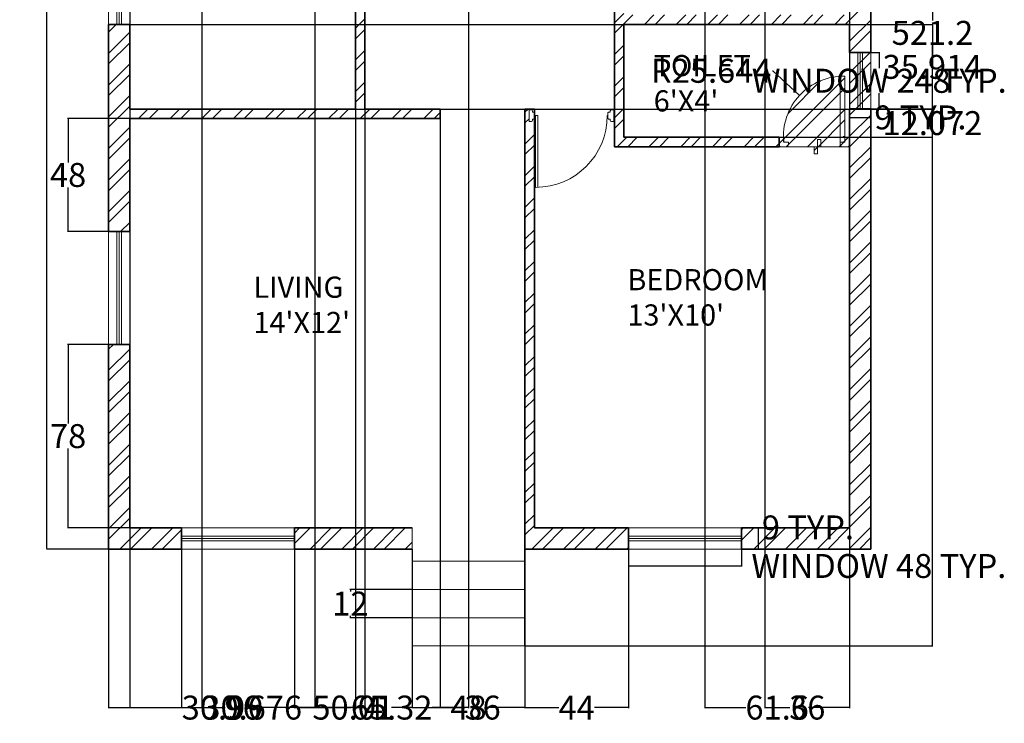
# Model space of a CAD drawing. Units: inches. Extents: x 2025 to 2472, y 2991 to 3578.
# Tile 1 of 2: x 2053 to 2472, y 2991 to 3291. Entities that reach past the tile are written whole.
import ezdxf

# ---------------------------------------------------------------- set-up
doc = ezdxf.new("R2010")
doc.units = ezdxf.units.IN
for name, color, linetype, lineweight in [('00 FURNITURE', 15, 'Continuous', 15), ('A-ANNO-DIMS', 2, 'Continuous', 18), ('A-AREA-IDEN', 7, 'Continuous', 18), ('A-DOOR', 4, 'Continuous', 18), ('A-FLOR-STRS', 7, 'Continuous', 18), ('A-WALL-PATT', 252, 'Continuous', 13), ('A_FUR 1', 5, 'Continuous', 5), ('WALL', 7, 'Continuous', 35), ('WINDOW', 160, 'Continuous', 13)]:
    doc.layers.add(name, color=color, linetype=linetype, lineweight=lineweight)
doc.styles.get("Standard").update_dxf_attribs({"font": 'arial.ttf'})
doc.dimstyles.get("Standard").update_dxf_attribs({"dimtxt": 10.18, "dimasz": 0.18, "dimexe": 0.18, "dimexo": 0.0625, "dimgap": 0.09, "dimtad": 0, "dimtih": 1, "dimtoh": 1, "dimdec": 0, "dimzin": 0, "dimdsep": 46, "dimlunit": 3, "dimtxsty": 'Standard', "dimcen": 0.09, "dimadec": 0, "dimazin": 0, "dimtfac": 1, "dimtdec": 0, "dimtofl": 0, "dimtmove": 0, "dimatfit": 3, "dimfxl": 1, "dimtolj": 1, "dimtzin": 0, "dimarcsym": 0})

# ---------------------------------------------------------------- blocks, each defined once
blk = doc.blocks.new('DDD')
at = {"layer": '00 FURNITURE'}
for p, q in [((-12579.77, -15859.53), (-12579.77, -15829.05)), ((-12578.77, -15859.53), (-12578.77, -15829.03)), ((-12612.02, -15857.03), (-12612.02, -15862.03)), ((-12611.02, -15857.03), (-12612.02, -15857.03)), ((-12610.52, -15858.03), (-12610.52, -15857.53)), ((-12577.52, -15858.03), (-12577.52, -15857.53)), ((-12577.02, -15857.03), (-12576.02, -15857.03)), ((-12576.02, -15857.03), (-12576.02, -15862.03)), ((-12610.52, -15861.53), (-12610.52, -15861.03)), ((-12578.77, -15859.53), (-12579.77, -15859.53)), ((-12577.52, -15861.53), (-12577.52, -15861.03)), ((-12612.02, -15862.03), (-12611.02, -15862.03)), ((-12576.02, -15862.03), (-12577.02, -15862.03))]:
    blk.add_line(p, q, dxfattribs=at)
for points in [[(-12610.52, -15861.03), (-12610.02, -15861.03, 0.414214), (-12609.52, -15860.53), (-12609.52, -15858.53, 0.414214), (-12610.02, -15858.03), (-12610.52, -15858.03)], [(-12577.52, -15861.03), (-12578.02, -15861.03, -0.414214), (-12578.52, -15860.53), (-12578.52, -15858.53, -0.414214), (-12578.02, -15858.03), (-12577.52, -15858.03)]]:
    blk.add_lwpolyline(points, format="xyb", dxfattribs=at)
for centre, radius, start, end in [((-12578.77, -15859.53), 30.5, 90, 180), ((-12611.02, -15857.53), 0.5, 0, 90), ((-12577.02, -15857.53), 0.5, 90, 180), ((-12611.02, -15861.53), 0.5, 270, 0), ((-12577.02, -15861.53), 0.5, 180, 270)]:
    blk.add_arc(centre, radius, start, end, dxfattribs=at)
blk = doc.blocks.new('ESTSET')
at = {"layer": 'A_FUR 1'}
for p, q in [((-10.44, 4.1), (-10.44, 32.1)), ((-8.44, 4.1), (-8.44, 32.1)), ((-36.44, 6.1), (-36.44, 3.1)), ((-34.44, 6.1), (-36.44, 6.1)), ((-34.44, 4.1), (-34.44, 6.1)), ((-34.44, 4.1), (-34.44, 6.1)), ((-8.44, 4.1), (-8.44, 6.1)), ((-8.44, 6.1), (-6.44, 6.1)), ((-8.44, 4.1), (-8.44, 6.1)), ((-6.44, 6.1), (-6.44, 3.1)), ((-6.44, 2.1), (-36.44, 2.1)), ((-35.44, 2.1), (-33.44, 2.1)), ((-32.44, 4.1), (-34.44, 4.1)), ((-32.44, 4.1), (-34.44, 4.1)), ((-32.44, 3.1), (-32.44, 4.1)), ((-10.44, 3.1), (-10.44, 4.1)), ((-10.44, 4.1), (-8.44, 4.1)), ((-10.44, 4.1), (-8.44, 4.1)), ((-7.44, 2.1), (-9.44, 2.1))]:
    blk.add_line(p, q, dxfattribs=at)
for points in [[(-21.44, 2.1), (-18.67, 2.1), (-18.67, 5.1), (-20.06, 5.1)], [(-20.06, 5.1), (-20.06, -0.91)], [(-21.44, 2.1), (-21.44, -0.91), (-20.06, -0.91)]]:
    blk.add_lwpolyline(points, dxfattribs=at)
for centre, radius, start, end in [((-8.91, 6.46), 25.64, 88.9606, 185.2816), ((-35.44, 3.1), 1, 180, 270), ((-33.44, 3.1), 1, 270, 0), ((-9.44, 3.1), 1, 180, 270), ((-7.44, 3.1), 1, 270, 0)]:
    blk.add_arc(centre, radius, start, end, dxfattribs=at)
blk = doc.blocks.new('WIN-48IN')
for p, q in [((48, 9), (0, 9)), ((48, 5.5), (0, 5.5)), ((48, 4.5), (0, 4.5)), ((48, 3.5), (0, 3.5)), ((0, 0), (48, 0))]:
    blk.add_line(p, q)
blk = doc.blocks.new('WIN-24IN')
for p, q in [((3.5, 24), (3.5, 0)), ((4.5, 24), (4.5, 0)), ((5.5, 24), (5.5, 0))]:
    blk.add_line(p, q)
blk.add_lwpolyline([(0, 0), (9, 0), (9, 24), (0, 24)], close=True)
blk = doc.blocks.new('*D6')
at = {"layer": 'A-ANNO-DIMS', "color": 0, "lineweight": -2, "transparency": 16777216}
for p, q in [((2311.79, 3065.44), (2311.79, 3058.12)), ((2359.79, 3065.44), (2359.79, 3058.12)), ((2311.97, 3058.3), (2359.61, 3058.3)), ((2359.79, 3058.3), (2359.97, 3058.3))]:
    blk.add_line(p, q, dxfattribs=at)
at = {"layer": 'A-ANNO-DIMS', "color": 0, "transparency": 16777216}
for points in [[(2311.97, 3058.33), (2311.97, 3058.27), (2311.79, 3058.3)], [(2359.61, 3058.33), (2359.61, 3058.27), (2359.79, 3058.3)]]:
    blk.add_solid(points, dxfattribs=at)
at = {"layer": 'Defpoints', "color": 0, "transparency": 16777216}
for p in [(2311.79, 3065.5), (2359.79, 3065.5), (2359.79, 3058.3)]:
    blk.add_point(p, dxfattribs=at)
at = {"layer": 'A-ANNO-DIMS', "color": 0, "transparency": 16777216, "insert": (2418.22, 3058.3), "char_height": 10.18, "attachment_point": 5}
blk.add_mtext('\\A1;WINDOW 48 TYP.', dxfattribs=at)
blk = doc.blocks.new('*D7')
at = {"layer": 'A-ANNO-DIMS', "color": 0, "lineweight": -2, "transparency": 16777216}
for p, q in [((2359.85, 3074.5), (2367.17, 3074.5)), ((2366.99, 3074.5), (2366.99, 3074.68)), ((2366.99, 3074.68), (2367.17, 3074.68)), ((2366.99, 3065.68), (2366.99, 3074.32)), ((2359.85, 3065.5), (2367.17, 3065.5))]:
    blk.add_line(p, q, dxfattribs=at)
at = {"layer": 'A-ANNO-DIMS', "color": 0, "transparency": 16777216}
for points in [[(2366.96, 3074.32), (2367.02, 3074.32), (2366.99, 3074.5)], [(2366.96, 3065.68), (2367.02, 3065.68), (2366.99, 3065.5)]]:
    blk.add_solid(points, dxfattribs=at)
at = {"layer": 'Defpoints', "color": 0, "transparency": 16777216}
for p in [(2359.79, 3074.5), (2366.99, 3074.5), (2359.79, 3065.5)]:
    blk.add_point(p, dxfattribs=at)
at = {"layer": 'A-ANNO-DIMS', "color": 0, "transparency": 16777216, "insert": (2388.08, 3074.68), "char_height": 10.18, "attachment_point": 5}
blk.add_mtext('\\A1;9 TYP.', dxfattribs=at)
blk = doc.blocks.new('*D8')
at = {"layer": 'A-ANNO-DIMS', "color": 0, "lineweight": -2, "transparency": 16777216}
for p, q in [((2414.85, 3276.57), (2418.57, 3276.57)), ((2418.39, 3276.39), (2418.39, 3269.93)), ((2418.39, 3252.75), (2418.39, 3259.22)), ((2414.85, 3252.57), (2418.57, 3252.57))]:
    blk.add_line(p, q, dxfattribs=at)
at = {"layer": 'A-ANNO-DIMS', "color": 0, "transparency": 16777216}
for points in [[(2418.36, 3276.39), (2418.42, 3276.39), (2418.39, 3276.57)], [(2418.36, 3252.75), (2418.42, 3252.75), (2418.39, 3252.57)]]:
    blk.add_solid(points, dxfattribs=at)
at = {"layer": 'Defpoints', "color": 0, "transparency": 16777216}
for p in [(2414.79, 3276.57), (2418.39, 3276.57), (2414.79, 3252.57)]:
    blk.add_point(p, dxfattribs=at)
at = {"layer": 'A-ANNO-DIMS', "color": 0, "transparency": 16777216, "insert": (2418.39, 3264.57), "char_height": 10.18, "attachment_point": 5}
blk.add_mtext('\\A1;WINDOW 24 TYP.', dxfattribs=at)
blk = doc.blocks.new('*D9')
at = {"layer": 'A-ANNO-DIMS', "color": 0, "lineweight": -2, "transparency": 16777216}
for p, q in [((2405.79, 3252.51), (2405.79, 3248.79)), ((2414.79, 3252.51), (2414.79, 3248.79)), ((2405.97, 3248.97), (2414.61, 3248.97)), ((2414.79, 3248.97), (2414.97, 3248.97))]:
    blk.add_line(p, q, dxfattribs=at)
at = {"layer": 'A-ANNO-DIMS', "color": 0, "transparency": 16777216}
for points in [[(2405.97, 3249), (2405.97, 3248.94), (2405.79, 3248.97)], [(2414.61, 3249), (2414.61, 3248.94), (2414.79, 3248.97)]]:
    blk.add_solid(points, dxfattribs=at)
at = {"layer": 'Defpoints', "color": 0, "transparency": 16777216}
for p in [(2405.79, 3252.57), (2414.79, 3252.57), (2414.79, 3248.97)]:
    blk.add_point(p, dxfattribs=at)
at = {"layer": 'A-ANNO-DIMS', "color": 0, "transparency": 16777216, "insert": (2435.88, 3248.97), "char_height": 10.18, "attachment_point": 5}
blk.add_mtext('\\A1;9 TYP.', dxfattribs=at)
blk = doc.blocks.new('*D15')
at = {"layer": 'A-ANNO-DIMS', "color": 0, "lineweight": -2, "transparency": 16777216}
for p, q in [((2414.85, 3545.5), (2441.17, 3545.5)), ((2440.99, 3545.32), (2440.99, 3290.19)), ((2440.99, 3024.48), (2440.99, 3279.61)), ((2267.85, 3024.3), (2441.17, 3024.3))]:
    blk.add_line(p, q, dxfattribs=at)
at = {"layer": 'A-ANNO-DIMS', "color": 0, "transparency": 16777216}
for points in [[(2440.96, 3545.32), (2441.02, 3545.32), (2440.99, 3545.5)], [(2440.96, 3024.48), (2441.02, 3024.48), (2440.99, 3024.3)]]:
    blk.add_solid(points, dxfattribs=at)
at = {"layer": 'Defpoints', "color": 0, "transparency": 16777216}
for p in [(2414.79, 3545.5), (2440.99, 3545.5), (2267.79, 3024.3)]:
    blk.add_point(p, dxfattribs=at)
at = {"layer": 'A-ANNO-DIMS', "color": 0, "transparency": 16777216, "insert": (2440.99, 3284.9), "char_height": 10.18, "attachment_point": 5}
blk.add_mtext('\\A1;521.2', dxfattribs=at)
blk = doc.blocks.new('*D16')
at = {"layer": 'A-ANNO-DIMS', "color": 0, "lineweight": -2, "transparency": 16777216}
for p, q in [((2090.72, 3545.5), (2064.41, 3545.5)), ((2064.59, 3545.32), (2064.59, 3310.79)), ((2064.59, 3065.68), (2064.59, 3300.21)), ((2090.72, 3065.5), (2064.41, 3065.5))]:
    blk.add_line(p, q, dxfattribs=at)
at = {"layer": 'A-ANNO-DIMS', "color": 0, "transparency": 16777216}
for points in [[(2064.56, 3545.32), (2064.62, 3545.32), (2064.59, 3545.5)], [(2064.56, 3065.68), (2064.62, 3065.68), (2064.59, 3065.5)]]:
    blk.add_solid(points, dxfattribs=at)
at = {"layer": 'Defpoints', "color": 0, "transparency": 16777216}
for p in [(2064.59, 3545.5), (2090.79, 3545.5), (2090.79, 3065.5)]:
    blk.add_point(p, dxfattribs=at)
at = {"layer": 'A-ANNO-DIMS', "color": 0, "transparency": 16777216, "insert": (2064.59, 3305.5), "char_height": 10.18, "attachment_point": 5}
blk.add_mtext('\\A1;480', dxfattribs=at)
blk = doc.blocks.new('*D17')
at = {"layer": 'A-ANNO-DIMS', "color": 0, "lineweight": -2, "transparency": 16777216}
for p, q in [((2219.79, 3024.24), (2219.79, 2997.92)), ((2267.79, 3024.24), (2267.79, 2997.92)), ((2219.97, 2998.1), (2236.19, 2998.1)), ((2267.61, 2998.1), (2251.38, 2998.1))]:
    blk.add_line(p, q, dxfattribs=at)
at = {"layer": 'A-ANNO-DIMS', "color": 0, "transparency": 16777216}
for points in [[(2219.97, 2998.13), (2219.97, 2998.07), (2219.79, 2998.1)], [(2267.61, 2998.13), (2267.61, 2998.07), (2267.79, 2998.1)]]:
    blk.add_solid(points, dxfattribs=at)
at = {"layer": 'Defpoints', "color": 0, "transparency": 16777216}
for p in [(2219.79, 3024.3), (2267.79, 3024.3), (2267.79, 2998.1)]:
    blk.add_point(p, dxfattribs=at)
at = {"layer": 'A-ANNO-DIMS', "color": 0, "transparency": 16777216, "insert": (2243.79, 2998.1), "char_height": 10.18, "attachment_point": 5}
blk.add_mtext('\\A1;48', dxfattribs=at)
blk = doc.blocks.new('*D18')
at = {"layer": 'A-ANNO-DIMS', "color": 0, "lineweight": -2, "transparency": 16777216}
for p, q in [((2099.79, 3536.44), (2099.79, 2997.92)), ((2130.46, 3536.44), (2130.46, 2997.92)), ((2099.97, 2998.1), (2130.28, 2998.1)), ((2130.46, 2998.1), (2130.64, 2998.1))]:
    blk.add_line(p, q, dxfattribs=at)
at = {"layer": 'A-ANNO-DIMS', "color": 0, "transparency": 16777216}
for points in [[(2099.97, 2998.13), (2099.97, 2998.07), (2099.79, 2998.1)], [(2130.28, 2998.13), (2130.28, 2998.07), (2130.46, 2998.1)]]:
    blk.add_solid(points, dxfattribs=at)
at = {"layer": 'Defpoints', "color": 0, "transparency": 16777216}
for p in [(2099.79, 3536.5), (2130.46, 3536.5), (2130.46, 2998.1)]:
    blk.add_point(p, dxfattribs=at)
at = {"layer": 'A-ANNO-DIMS', "color": 0, "transparency": 16777216, "insert": (2151.86, 2998.1), "char_height": 10.18, "attachment_point": 5}
blk.add_mtext('\\A1;30.676', dxfattribs=at)
blk = doc.blocks.new('*D19')
at = {"layer": 'A-ANNO-DIMS', "color": 0, "lineweight": -2, "transparency": 16777216}
for p, q in [((2178.46, 3536.44), (2178.46, 2997.92)), ((2243.79, 3536.44), (2243.79, 2997.92)), ((2178.64, 2998.1), (2193.88, 2998.1)), ((2243.61, 2998.1), (2228.37, 2998.1))]:
    blk.add_line(p, q, dxfattribs=at)
at = {"layer": 'A-ANNO-DIMS', "color": 0, "transparency": 16777216}
for points in [[(2178.64, 2998.13), (2178.64, 2998.07), (2178.46, 2998.1)], [(2243.61, 2998.13), (2243.61, 2998.07), (2243.79, 2998.1)]]:
    blk.add_solid(points, dxfattribs=at)
at = {"layer": 'Defpoints', "color": 0, "transparency": 16777216}
for p in [(2178.46, 3536.5), (2243.79, 3536.5), (2243.79, 2998.1)]:
    blk.add_point(p, dxfattribs=at)
at = {"layer": 'A-ANNO-DIMS', "color": 0, "transparency": 16777216, "insert": (2211.12, 2998.1), "char_height": 10.18, "attachment_point": 5}
blk.add_mtext('\\A1;65.32', dxfattribs=at)
blk = doc.blocks.new('*D20')
at = {"layer": 'A-ANNO-DIMS', "color": 0, "lineweight": -2, "transparency": 16777216}
for p, q in [((2344.19, 3536.44), (2344.19, 2997.92)), ((2405.79, 3536.44), (2405.79, 2997.92)), ((2344.37, 2998.1), (2361.65, 2998.1)), ((2405.61, 2998.1), (2388.32, 2998.1))]:
    blk.add_line(p, q, dxfattribs=at)
at = {"layer": 'A-ANNO-DIMS', "color": 0, "transparency": 16777216}
for points in [[(2344.37, 2998.13), (2344.37, 2998.07), (2344.19, 2998.1)], [(2405.61, 2998.13), (2405.61, 2998.07), (2405.79, 2998.1)]]:
    blk.add_solid(points, dxfattribs=at)
at = {"layer": 'Defpoints', "color": 0, "transparency": 16777216}
for p in [(2344.19, 3536.5), (2405.79, 3536.5), (2405.79, 2998.1)]:
    blk.add_point(p, dxfattribs=at)
at = {"layer": 'A-ANNO-DIMS', "color": 0, "transparency": 16777216, "insert": (2374.99, 2998.1), "char_height": 10.18, "attachment_point": 5}
blk.add_mtext('\\A1;61.6', dxfattribs=at)
blk = doc.blocks.new('*D21')
at = {"layer": 'A-ANNO-DIMS', "color": 0, "lineweight": -2, "transparency": 16777216}
for p, q in [((2090.79, 3065.44), (2090.79, 2997.92)), ((2121.78, 3065.44), (2121.78, 2997.92)), ((2090.97, 2998.1), (2121.6, 2998.1)), ((2121.78, 2998.1), (2121.96, 2998.1))]:
    blk.add_line(p, q, dxfattribs=at)
at = {"layer": 'A-ANNO-DIMS', "color": 0, "transparency": 16777216}
for points in [[(2090.97, 2998.13), (2090.97, 2998.07), (2090.79, 2998.1)], [(2121.6, 2998.13), (2121.6, 2998.07), (2121.78, 2998.1)]]:
    blk.add_solid(points, dxfattribs=at)
at = {"layer": 'Defpoints', "color": 0, "transparency": 16777216}
for p in [(2090.79, 3065.5), (2121.78, 3065.5), (2121.78, 2998.1)]:
    blk.add_point(p, dxfattribs=at)
at = {"layer": 'A-ANNO-DIMS', "color": 0, "transparency": 16777216, "insert": (2139.23, 2998.1), "char_height": 10.18, "attachment_point": 5}
blk.add_mtext('\\A1;30.99', dxfattribs=at)
blk = doc.blocks.new('*D22')
at = {"layer": 'A-ANNO-DIMS', "color": 0, "lineweight": -2, "transparency": 16777216}
for p, q in [((2169.78, 3065.44), (2169.78, 2997.92)), ((2219.79, 3065.44), (2219.79, 2997.92)), ((2169.96, 2998.1), (2178.5, 2998.1)), ((2219.61, 2998.1), (2211.06, 2998.1))]:
    blk.add_line(p, q, dxfattribs=at)
at = {"layer": 'A-ANNO-DIMS', "color": 0, "transparency": 16777216}
for points in [[(2169.96, 2998.13), (2169.96, 2998.07), (2169.78, 2998.1)], [(2219.61, 2998.13), (2219.61, 2998.07), (2219.79, 2998.1)]]:
    blk.add_solid(points, dxfattribs=at)
at = {"layer": 'Defpoints', "color": 0, "transparency": 16777216}
for p in [(2169.78, 3065.5), (2219.79, 3065.5), (2219.79, 2998.1)]:
    blk.add_point(p, dxfattribs=at)
at = {"layer": 'A-ANNO-DIMS', "color": 0, "transparency": 16777216, "insert": (2194.78, 2998.1), "char_height": 10.18, "attachment_point": 5}
blk.add_mtext('\\A1;50.01', dxfattribs=at)
blk = doc.blocks.new('*D23')
at = {"layer": 'A-ANNO-DIMS', "color": 0, "lineweight": -2, "transparency": 16777216}
for p, q in [((2267.79, 3065.44), (2267.79, 2997.92)), ((2311.79, 3065.44), (2311.79, 2997.92)), ((2267.97, 2998.1), (2282.22, 2998.1)), ((2311.61, 2998.1), (2297.35, 2998.1))]:
    blk.add_line(p, q, dxfattribs=at)
at = {"layer": 'A-ANNO-DIMS', "color": 0, "transparency": 16777216}
for points in [[(2267.97, 2998.13), (2267.97, 2998.07), (2267.79, 2998.1)], [(2311.61, 2998.13), (2311.61, 2998.07), (2311.79, 2998.1)]]:
    blk.add_solid(points, dxfattribs=at)
at = {"layer": 'Defpoints', "color": 0, "transparency": 16777216}
for p in [(2267.79, 3065.5), (2311.79, 3065.5), (2311.79, 2998.1)]:
    blk.add_point(p, dxfattribs=at)
at = {"layer": 'A-ANNO-DIMS', "color": 0, "transparency": 16777216, "insert": (2289.79, 2998.1), "char_height": 10.18, "attachment_point": 5}
blk.add_mtext('\\A1;44', dxfattribs=at)
blk = doc.blocks.new('*D24')
at = {"layer": 'A-ANNO-DIMS', "color": 0, "lineweight": -2, "transparency": 16777216}
for p, q in [((2099.72, 3152.5), (2073.41, 3152.5)), ((2073.59, 3152.32), (2073.59, 3118.79)), ((2073.59, 3074.68), (2073.59, 3108.21)), ((2099.72, 3074.5), (2073.41, 3074.5))]:
    blk.add_line(p, q, dxfattribs=at)
at = {"layer": 'A-ANNO-DIMS', "color": 0, "transparency": 16777216}
for points in [[(2073.56, 3152.32), (2073.62, 3152.32), (2073.59, 3152.5)], [(2073.56, 3074.68), (2073.62, 3074.68), (2073.59, 3074.5)]]:
    blk.add_solid(points, dxfattribs=at)
at = {"layer": 'Defpoints', "color": 0, "transparency": 16777216}
for p in [(2073.59, 3152.5), (2099.79, 3152.5), (2099.79, 3074.5)]:
    blk.add_point(p, dxfattribs=at)
at = {"layer": 'A-ANNO-DIMS', "color": 0, "transparency": 16777216, "insert": (2073.59, 3113.5), "char_height": 10.18, "attachment_point": 5}
blk.add_mtext('\\A1;78', dxfattribs=at)
blk = doc.blocks.new('*D25')
at = {"layer": 'A-ANNO-DIMS', "color": 0, "lineweight": -2, "transparency": 16777216}
for p, q in [((2099.72, 3248.5), (2073.41, 3248.5)), ((2073.59, 3248.32), (2073.59, 3229.79)), ((2073.59, 3200.68), (2073.59, 3219.21)), ((2099.72, 3200.5), (2073.41, 3200.5))]:
    blk.add_line(p, q, dxfattribs=at)
at = {"layer": 'A-ANNO-DIMS', "color": 0, "transparency": 16777216}
for points in [[(2073.56, 3248.32), (2073.62, 3248.32), (2073.59, 3248.5)], [(2073.56, 3200.68), (2073.62, 3200.68), (2073.59, 3200.5)]]:
    blk.add_solid(points, dxfattribs=at)
at = {"layer": 'Defpoints', "color": 0, "transparency": 16777216}
for p in [(2073.59, 3248.5), (2099.79, 3248.5), (2099.79, 3200.5)]:
    blk.add_point(p, dxfattribs=at)
at = {"layer": 'A-ANNO-DIMS', "color": 0, "transparency": 16777216, "insert": (2073.59, 3224.5), "char_height": 10.18, "attachment_point": 5}
blk.add_mtext('\\A1;48', dxfattribs=at)
blk = doc.blocks.new('*D27')
at = {"layer": 'A-ANNO-DIMS', "color": 0, "lineweight": -2, "transparency": 16777216}
for p, q in [((2099.85, 3288.42), (2441.17, 3288.42)), ((2440.99, 3288.24), (2440.99, 3275.75)), ((2440.99, 3252.68), (2440.99, 3265.17)), ((2099.85, 3252.5), (2441.17, 3252.5))]:
    blk.add_line(p, q, dxfattribs=at)
at = {"layer": 'A-ANNO-DIMS', "color": 0, "transparency": 16777216}
for points in [[(2440.96, 3288.24), (2441.02, 3288.24), (2440.99, 3288.42)], [(2440.96, 3252.68), (2441.02, 3252.68), (2440.99, 3252.5)]]:
    blk.add_solid(points, dxfattribs=at)
at = {"layer": 'Defpoints', "color": 0, "transparency": 16777216}
for p in [(2099.79, 3288.42), (2440.99, 3288.42), (2099.79, 3252.5)]:
    blk.add_point(p, dxfattribs=at)
at = {"layer": 'A-ANNO-DIMS', "color": 0, "transparency": 16777216, "insert": (2440.99, 3270.46), "char_height": 10.18, "attachment_point": 5}
blk.add_mtext('\\A1;35.914', dxfattribs=at)
blk = doc.blocks.new('*D30')
at = {"layer": 'A-ANNO-DIMS', "color": 0, "lineweight": -2, "transparency": 16777216}
for p, q in [((2414.85, 3252.57), (2441.17, 3252.57)), ((2440.99, 3252.39), (2440.99, 3251.83)), ((2405.82, 3240.5), (2441.17, 3240.5)), ((2440.99, 3240.68), (2440.99, 3241.25))]:
    blk.add_line(p, q, dxfattribs=at)
at = {"layer": 'A-ANNO-DIMS', "color": 0, "transparency": 16777216}
for points in [[(2440.96, 3252.39), (2441.02, 3252.39), (2440.99, 3252.57)], [(2440.96, 3240.68), (2441.02, 3240.68), (2440.99, 3240.5)]]:
    blk.add_solid(points, dxfattribs=at)
at = {"layer": 'Defpoints', "color": 0, "transparency": 16777216}
for p in [(2414.79, 3252.57), (2405.75, 3240.5), (2440.99, 3240.5)]:
    blk.add_point(p, dxfattribs=at)
at = {"layer": 'A-ANNO-DIMS', "color": 0, "transparency": 16777216, "insert": (2440.99, 3246.54), "char_height": 10.18, "attachment_point": 5}
blk.add_mtext('\\A1;12.072', dxfattribs=at)
blk = doc.blocks.new('*D31')
at = {"layer": 'A-ANNO-DIMS', "color": 0, "lineweight": -2, "transparency": 16777216}
for p, q in [((2099.79, 3412.44), (2099.79, 2997.92)), ((2195.79, 3412.44), (2195.79, 2997.92)), ((2099.97, 2998.1), (2140.41, 2998.1)), ((2195.61, 2998.1), (2155.16, 2998.1))]:
    blk.add_line(p, q, dxfattribs=at)
at = {"layer": 'A-ANNO-DIMS', "color": 0, "transparency": 16777216}
for points in [[(2099.97, 2998.13), (2099.97, 2998.07), (2099.79, 2998.1)], [(2195.61, 2998.13), (2195.61, 2998.07), (2195.79, 2998.1)]]:
    blk.add_solid(points, dxfattribs=at)
at = {"layer": 'Defpoints', "color": 0, "transparency": 16777216}
for p in [(2099.79, 3412.5), (2195.79, 3412.5), (2195.79, 2998.1)]:
    blk.add_point(p, dxfattribs=at)
at = {"layer": 'A-ANNO-DIMS', "color": 0, "transparency": 16777216, "insert": (2147.79, 2998.1), "char_height": 10.18, "attachment_point": 5}
blk.add_mtext('\\A1;96', dxfattribs=at)
blk = doc.blocks.new('*D35')
at = {"layer": 'A-ANNO-DIMS', "color": 0, "lineweight": -2, "transparency": 16777216}
for p, q in [((2309.85, 3288.5), (2441.17, 3288.5)), ((2440.99, 3288.32), (2440.99, 3269.79)), ((2440.99, 3240.68), (2440.99, 3259.21)), ((2309.85, 3240.5), (2441.17, 3240.5))]:
    blk.add_line(p, q, dxfattribs=at)
at = {"layer": 'A-ANNO-DIMS', "color": 0, "transparency": 16777216}
for points in [[(2440.96, 3288.32), (2441.02, 3288.32), (2440.99, 3288.5)], [(2440.96, 3240.68), (2441.02, 3240.68), (2440.99, 3240.5)]]:
    blk.add_solid(points, dxfattribs=at)
at = {"layer": 'Defpoints', "color": 0, "transparency": 16777216}
for p in [(2309.79, 3288.5), (2440.99, 3288.5), (2309.79, 3240.5)]:
    blk.add_point(p, dxfattribs=at)
at = {"layer": 'A-ANNO-DIMS', "color": 0, "transparency": 16777216, "insert": (2440.99, 3264.5), "char_height": 10.18, "attachment_point": 5}
blk.add_mtext('\\A1;48', dxfattribs=at)
blk = doc.blocks.new('*D38')
at = {"layer": 'A-ANNO-DIMS', "color": 0, "lineweight": -2, "transparency": 16777216}
for p, q in [((2267.79, 3252.44), (2267.79, 2997.92)), ((2231.79, 3248.44), (2231.79, 2997.92)), ((2231.97, 2998.1), (2242.41, 2998.1)), ((2267.61, 2998.1), (2257.16, 2998.1))]:
    blk.add_line(p, q, dxfattribs=at)
at = {"layer": 'A-ANNO-DIMS', "color": 0, "transparency": 16777216}
for points in [[(2231.97, 2998.13), (2231.97, 2998.07), (2231.79, 2998.1)], [(2267.61, 2998.13), (2267.61, 2998.07), (2267.79, 2998.1)]]:
    blk.add_solid(points, dxfattribs=at)
at = {"layer": 'Defpoints', "color": 0, "transparency": 16777216}
for p in [(2267.79, 3252.5), (2231.79, 3248.5), (2267.79, 2998.1)]:
    blk.add_point(p, dxfattribs=at)
at = {"layer": 'A-ANNO-DIMS', "color": 0, "transparency": 16777216, "insert": (2249.79, 2998.1), "char_height": 10.18, "attachment_point": 5}
blk.add_mtext('\\A1;36', dxfattribs=at)
blk = doc.blocks.new('*D41')
at = {"layer": 'A-ANNO-DIMS', "color": 0, "lineweight": -2, "transparency": 16777216}
for p, q in [((2195.79, 3360.44), (2195.79, 2997.92)), ((2199.79, 3338.9), (2199.79, 2997.92)), ((2195.97, 2998.1), (2199.61, 2998.1)), ((2199.79, 2998.1), (2199.97, 2998.1))]:
    blk.add_line(p, q, dxfattribs=at)
at = {"layer": 'A-ANNO-DIMS', "color": 0, "transparency": 16777216}
for points in [[(2195.97, 2998.13), (2195.97, 2998.07), (2195.79, 2998.1)], [(2199.61, 2998.13), (2199.61, 2998.07), (2199.79, 2998.1)]]:
    blk.add_solid(points, dxfattribs=at)
at = {"layer": 'Defpoints', "color": 0, "transparency": 16777216}
for p in [(2195.79, 3360.5), (2199.79, 3338.96), (2199.79, 2998.1)]:
    blk.add_point(p, dxfattribs=at)
at = {"layer": 'A-ANNO-DIMS', "color": 0, "transparency": 16777216, "insert": (2203.58, 2998.1), "char_height": 10.18, "attachment_point": 5}
blk.add_mtext('\\A1;4', dxfattribs=at)
blk = doc.blocks.new('*D42')
at = {"layer": 'A-ANNO-DIMS', "color": 0, "lineweight": -2, "transparency": 16777216}
for p, q in [((2369.79, 3328.44), (2369.79, 2997.92)), ((2405.79, 3328.44), (2405.79, 2997.92)), ((2369.97, 2998.1), (2380.41, 2998.1)), ((2405.61, 2998.1), (2395.16, 2998.1))]:
    blk.add_line(p, q, dxfattribs=at)
at = {"layer": 'A-ANNO-DIMS', "color": 0, "transparency": 16777216}
for points in [[(2369.97, 2998.13), (2369.97, 2998.07), (2369.79, 2998.1)], [(2405.61, 2998.13), (2405.61, 2998.07), (2405.79, 2998.1)]]:
    blk.add_solid(points, dxfattribs=at)
at = {"layer": 'Defpoints', "color": 0, "transparency": 16777216}
for p in [(2369.79, 3328.5), (2405.79, 3328.5), (2405.79, 2998.1)]:
    blk.add_point(p, dxfattribs=at)
at = {"layer": 'A-ANNO-DIMS', "color": 0, "transparency": 16777216, "insert": (2387.79, 2998.1), "char_height": 10.18, "attachment_point": 5}
blk.add_mtext('\\A1;36', dxfattribs=at)
blk = doc.blocks.new('*D44')
at = {"layer": 'A-ANNO-DIMS', "color": 0, "lineweight": -2, "transparency": 16777216}
for p, q in [((2219.72, 3048.3), (2193.41, 3048.3)), ((2193.59, 3048.12), (2193.59, 3047.5)), ((2219.72, 3036.3), (2193.41, 3036.3)), ((2193.59, 3036.48), (2193.59, 3037.1))]:
    blk.add_line(p, q, dxfattribs=at)
at = {"layer": 'A-ANNO-DIMS', "color": 0, "transparency": 16777216}
for points in [[(2193.56, 3048.12), (2193.62, 3048.12), (2193.59, 3048.3)], [(2193.56, 3036.48), (2193.62, 3036.48), (2193.59, 3036.3)]]:
    blk.add_solid(points, dxfattribs=at)
at = {"layer": 'Defpoints', "color": 0, "transparency": 16777216}
for p in [(2193.59, 3048.3), (2219.79, 3048.3), (2219.79, 3036.3)]:
    blk.add_point(p, dxfattribs=at)
at = {"layer": 'A-ANNO-DIMS', "color": 0, "transparency": 16777216, "insert": (2193.59, 3042.3), "char_height": 10.18, "attachment_point": 5}
blk.add_mtext('\\A1;12', dxfattribs=at)
blk = doc.blocks.new('*D46')
at = {"layer": 'A-ANNO-DIMS', "color": 0, "lineweight": -2, "transparency": 16777216}
for p, q in [((2373.04, 3268.78), (2373.22, 3268.78)), ((2373.22, 3268.78), (2384.37, 3258.43)), ((2403.2, 3240.86), (2403.38, 3240.86)), ((2403.29, 3240.77), (2403.29, 3240.95))]:
    blk.add_line(p, q, dxfattribs=at)
at = {"layer": 'A-ANNO-DIMS', "color": 0, "transparency": 16777216}
blk.add_solid([(2384.39, 3258.46), (2384.35, 3258.41), (2384.5, 3258.31)], dxfattribs=at)
at = {"layer": 'Defpoints', "color": 0, "transparency": 16777216}
for p in [(2384.5, 3258.31), (2403.29, 3240.86)]:
    blk.add_point(p, dxfattribs=at)
at = {"layer": 'A-ANNO-DIMS', "color": 0, "transparency": 16777216, "insert": (2346.97, 3268.78), "char_height": 10.18, "attachment_point": 5}
blk.add_mtext('\\A1;R25.644', dxfattribs=at)

msp = doc.modelspace()

# ---------------------------------------------------------------- hatches: boundary and pattern name
at = {"layer": 'A-WALL-PATT'}
h = msp.add_hatch(dxfattribs=at)
h.set_pattern_fill('ANSI32', color=256)
h.paths.add_polyline_path([(2130.4623, 3545.5019), (2090.7862, 3545.5019), (2090.7862, 3399.5018), (2099.7862, 3399.5018), (2099.7862, 3412.5019), (2195.7862, 3412.5019), (2195.7862, 3394.5019), (2199.7862, 3394.5019), (2199.7862, 3412.5019), (2207.7862, 3412.5019), (2207.7862, 3416.5019), (2099.7862, 3416.5019), (2099.7862, 3536.5019), (2130.4623, 3536.5019)])
h.paths.add_polyline_path([(2296.1871, 3545.5019), (2296.187, 3545.5019), (2178.4623, 3545.5019), (2178.4623, 3536.5019), (2243.7862, 3536.5019), (2243.7862, 3417.5019), (2243.7862, 3417.5019), (2243.7862, 3412.5019), (2247.7862, 3412.5019), (2247.7862, 3536.5019), (2296.1871, 3536.5019)])
h.paths.add_polyline_path([(2305.7862, 3236.5019), (2305.7862, 3247.2334), (2305.5512, 3247.2334), (2305.5512, 3252.2334), (2305.7862, 3295.8929), (2309.7862, 3295.8929), (2309.7862, 3292.5019), (2405.7862, 3292.5019), (2405.7862, 3328.5019), (2369.7862, 3328.5019), (2369.7862, 3376.5019), (2309.7862, 3376.5019), (2309.7862, 3355.8929), (2305.7862, 3355.8929), (2305.7862, 3412.5019), (2283.7862, 3412.5019), (2282.7862, 3412.502, -0.41421356), (2282.2862, 3413.002), (2282.2862, 3413.502), (2281.7862, 3413.502, -0.41421356), (2281.2862, 3414.002), (2281.0362, 3415.002, 0.40464108), (2251.5362, 3445.4856), (2251.5362, 3415.002), (2250.2862, 3415.002), (2250.2862, 3414.002, -0.41421356), (2249.7862, 3413.502), (2249.2862, 3413.502), (2249.2862, 3413.002, -0.41421356), (2248.7862, 3412.502), (2247.7862, 3412.502), (2247.7862, 3417.502), (2248.7862, 3417.502, -0.41421356), (2249.2862, 3417.002), (2249.2862, 3416.502), (2249.7862, 3416.502, -0.41421356), (2250.2862, 3416.002), (2250.5362, 3445.502, -0.40734559), (2281.2864, 3415.986, -0.42361429), (2281.7862, 3416.502), (2282.2862, 3416.502), (2282.2862, 3417.002, -0.41421356), (2282.7862, 3417.502), (2283.7862, 3417.502), (2283.7862, 3416.5019), (2405.7862, 3416.5019), (2405.7862, 3536.5019), (2344.1871, 3536.5019), (2344.1871, 3545.5019), (2414.7862, 3545.5019), (2414.7862, 3276.5742), (2414.7861, 3252.5742), (2405.7861, 3252.5742), (2405.7861, 3276.5742), (2405.7862, 3288.5019), (2309.7862, 3288.5019), (2309.7862, 3240.5019), (2375.7543, 3240.5019), (2375.7543, 3240.5021), (2377.648, 3240.5021, -0.42367667), (2403.7543, 3266.5021), (2403.7543, 3240.5021), (2405.7543, 3240.5021), (2405.7543, 3237.5021, -0.41421356), (2404.7543, 3236.5021), (2402.7543, 3236.5021), (2392.14, 3236.5021), (2392.14, 3233.4968), (2390.7543, 3233.4968), (2390.7543, 3236.5021), (2375.7862, 3236.5021), (2375.7862, 3236.5019)])
h.paths.add_polyline_path([(2414.7862, 3252.5742), (2405.7862, 3252.5742), (2405.7862, 3236.5019), (2405.7862, 3074.5019), (2359.7872, 3074.5019), (2359.7872, 3065.5019), (2414.7862, 3065.5019)])
h.paths.add_polyline_path([(2311.7872, 3074.5019), (2311.7872, 3074.5019), (2271.7862, 3074.5019), (2271.7862, 3248.2334), (2271.0512, 3248.2334), (2271.0512, 3247.7334, -0.41421356), (2270.5512, 3247.2334), (2269.5512, 3247.2334), (2269.5512, 3252.5019), (2267.7862, 3252.5019), (2267.7862, 3065.5019), (2311.7872, 3065.5019)])
h.paths.add_polyline_path([(2219.7862, 3074.5019), (2169.7756, 3074.5019), (2169.7756, 3065.502), (2169.7756, 3065.502), (2219.7862, 3065.5019)])
h.paths.add_polyline_path([(2121.7756, 3074.5019), (2099.7862, 3074.5019), (2099.7862, 3152.4991), (2090.7862, 3152.4991), (2090.7862, 3065.5019), (2121.7756, 3065.5019)])
h.paths.add_polyline_path([(2099.7862, 3248.5019), (2231.7862, 3248.5019), (2231.7862, 3252.5019), (2199.7862, 3252.5019), (2199.7862, 3302.9583), (2195.7862, 3302.9583), (2195.7862, 3252.5019), (2099.7862, 3252.5019), (2099.7862, 3288.4156), (2090.7862, 3288.4156), (2090.7862, 3200.4991), (2099.7862, 3200.4991), (2099.7862, 3200.4991)])
h.paths.add_polyline_path([(2099.7862, 3375.5018), (2090.7862, 3375.5018), (2090.7862, 3336.4156), (2099.7862, 3336.4156), (2099.7862, 3336.4156), (2099.7862, 3360.5019), (2195.7862, 3360.5019), (2195.7862, 3338.9583), (2199.7862, 3338.9583), (2199.7862, 3364.5019), (2099.7862, 3364.5019)])

# ---------------------------------------------------------------- linework, layer by layer
at = {"layer": 'A-FLOR-STRS'}
for p, q in [((2219.7862, 3024.3023), (2219.7862, 3074.5019)), ((2219.7862, 3060.3023), (2267.7862, 3060.3023)), ((2219.7862, 3048.3023), (2267.7862, 3048.3023)), ((2219.7862, 3036.3023), (2267.7862, 3036.3023)), ((2219.7862, 3024.3023), (2267.7862, 3024.3023))]:
    msp.add_line(p, q, dxfattribs=at)
at = {"layer": 'WALL'}
for p, q in [((2414.7862, 3545.5019), (2414.7862, 3276.5742)), ((2195.7862, 3252.5019), (2195.7862, 3302.9583)), ((2199.7862, 3252.5019), (2199.7862, 3302.9583)), ((2305.7862, 3295.8929), (2305.7862, 3236.5019)), ((2099.7862, 3288.4156), (2090.7862, 3288.4156)), ((2090.7862, 3200.4991), (2090.7862, 3288.4156)), ((2099.7862, 3252.5019), (2099.7862, 3288.4156)), ((2309.7862, 3288.5019), (2405.7862, 3288.5019)), ((2309.7862, 3288.5019), (2309.7862, 3240.5019)), ((2405.7862, 3288.5019), (2405.7862, 3276.5742)), ((2405.7862, 3276.5742), (2414.7862, 3276.5742)), ((2099.7862, 3252.5019), (2195.7862, 3252.5019)), ((2199.7862, 3252.5019), (2231.7862, 3252.5019)), ((2231.7862, 3248.5019), (2231.7862, 3252.5019)), ((2267.7862, 3024.3023), (2267.7862, 3252.5019)), ((2267.7862, 3252.5019), (2271.7862, 3252.5019)), ((2271.7862, 3074.5019), (2271.7862, 3252.5019)), ((2405.7862, 3252.5742), (2414.7862, 3252.5742)), ((2405.7862, 3252.5742), (2405.7862, 3236.5019)), ((2414.7862, 3252.5742), (2414.7862, 3065.5019)), ((2099.7862, 3248.5019), (2231.7862, 3248.5019)), ((2099.7862, 3200.4991), (2099.7862, 3248.5019)), ((2309.7862, 3240.5019), (2375.7862, 3240.5019)), ((2375.7862, 3240.5019), (2375.7862, 3236.5019)), ((2305.7862, 3236.5019), (2375.7862, 3236.5019)), ((2405.7862, 3236.5019), (2405.7862, 3074.5019)), ((2099.7862, 3200.4991), (2090.7862, 3200.4991)), ((2090.7862, 3065.5019), (2090.7862, 3152.4991)), ((2099.7862, 3152.4991), (2090.7862, 3152.4991)), ((2099.7862, 3074.5019), (2099.7862, 3152.4991)), ((2121.7756, 3074.5019), (2099.7862, 3074.5019)), ((2121.7756, 3074.5019), (2121.7756, 3065.5019)), ((2219.7862, 3074.5019), (2169.7756, 3074.5019)), ((2169.7756, 3074.5019), (2169.7756, 3065.5019)), ((2311.7872, 3074.5019), (2271.7862, 3074.5019)), ((2311.7872, 3074.5019), (2311.7872, 3065.5019)), ((2405.7862, 3074.5019), (2359.7872, 3074.5019)), ((2359.7872, 3074.5019), (2359.7872, 3065.5019)), ((2121.7756, 3065.5019), (2090.7862, 3065.5019)), ((2219.7862, 3065.5019), (2169.7756, 3065.5019)), ((2311.7872, 3065.5019), (2267.7862, 3065.5019)), ((2414.7862, 3065.5019), (2359.7872, 3065.5019))]:
    msp.add_line(p, q, dxfattribs=at)

# ---------------------------------------------------------------- block references
at = {"layer": 'A-DOOR'}
msp.add_blockref('ESTSET', (2412.1979, 3234.4055), dxfattribs=at)
at = {"layer": 'A-DOOR', "rotation": 180}
msp.add_blockref('DDD', (-10306.4722, -12609.7956), dxfattribs=at)
at = {"layer": 'WINDOW'}
for p, rotation in [((2090.7862, 3336.416), 270.0000000000012), ((2090.7862, 3200.4994), 270.0000000000007)]:
    msp.add_blockref('WIN-48IN', p, dxfattribs=dict(at, rotation=rotation))
for name, p in [('WIN-24IN', (2405.786, 3252.574)), ('WIN-48IN', (2121.7753, 3065.502)), ('WIN-48IN', (2311.7869, 3065.502))]:
    msp.add_blockref(name, p, dxfattribs=at)

# ---------------------------------------------------------------- texts
at = {"layer": 'A-AREA-IDEN', "char_height": 9, "attachment_point": 1}
for s, insert in [("TOILET\\P6'X4'", (2322.5154, 3275.4852)), ("LIVING \\P14'X12'", (2152.3549, 3181.2936)), ("BEDROOM\\P13'X10'", (2311.3312, 3184.4865))]:
    msp.add_mtext_dynamic_manual_height_columns(s, width=96.486866, gutter_width=12.5, heights=[0], dxfattribs=dict(at, insert=insert))

# ---------------------------------------------------------------- dimensions: what is measured, and where the dimension line sits
at = {"layer": 'A-ANNO-DIMS'}
for base, p1, p2, angle, override, picture, middle in [((2064.5861, 3545.5019), (2090.7862, 3065.5019), (2090.7862, 3545.5019), 90, {"dimdec": 0, "dimlfac": 1, "dimrnd": 0, "dimzin": 0, "dimdsep": 46, "dimlunit": 2}, '*D16', (2064.5861, 3305.5019)), ((2440.9862, 3545.5019), (2267.7862, 3024.3023), (2414.7862, 3545.5019), 90, {"dimdec": 1, "dimlfac": 1, "dimrnd": 0, "dimzin": 0, "dimdsep": 46, "dimlunit": 2}, '*D15', (2440.9862, 3284.9021)), ((2440.9862, 3288.4156), (2099.7862, 3252.5019), (2099.7862, 3288.4156), 90, {"dimdec": 3, "dimlfac": 1, "dimrnd": 0, "dimzin": 0, "dimdsep": 46, "dimlunit": 2}, '*D27', (2440.9862, 3270.4588)), ((2440.9862, 3288.5019), (2309.7862, 3240.5019), (2309.7862, 3288.5019), 90, {"dimdec": 0, "dimlfac": 1, "dimrnd": 0, "dimzin": 0, "dimdsep": 46, "dimlunit": 2}, '*D35', (2440.9862, 3264.5019)), ((2440.9862, 3240.5021), (2414.7862, 3252.5742), (2405.7543, 3240.5021), 90, {"dimdec": 3, "dimlfac": 1, "dimrnd": 0, "dimzin": 0, "dimdsep": 46, "dimlunit": 2}, '*D30', (2440.9862, 3246.5381)), ((2073.5862, 3248.5019), (2099.7862, 3200.4991), (2099.7862, 3248.5019), 89.999993, {"dimdec": 0, "dimlfac": 1, "dimrnd": 0, "dimzin": 0, "dimdsep": 46, "dimlunit": 2}, '*D25', (2073.5862, 3224.5005)), ((2073.5862, 3152.4991), (2099.7862, 3074.5019), (2099.7862, 3152.4991), 90.000005, {"dimdec": 0, "dimlfac": 1, "dimrnd": 0, "dimzin": 0, "dimdsep": 46, "dimlunit": 2}, '*D24', (2073.5862, 3113.5005)), ((2193.5862, 3048.3023), (2219.7862, 3036.3023), (2219.7862, 3048.3023), 90, {"dimdec": 0, "dimlfac": 1, "dimrnd": 0, "dimzin": 0, "dimdsep": 46, "dimlunit": 2}, '*D44', (2193.5862, 3042.3023))]:
    dim = msp.add_linear_dim(base=base, p1=p1, p2=p2, angle=angle, dimstyle='Standard', override=override, dxfattribs=at)
    dim.commit()
    dim.dimension.update_dxf_attribs({"geometry": picture, "text_midpoint": middle})
for base, p1, p2, override, picture, middle in [((2130.4623, 2998.1023), (2099.7862, 3536.5019), (2130.4623, 3536.5019), {"dimdec": 3, "dimlfac": 1, "dimrnd": 0, "dimzin": 0, "dimdsep": 46, "dimlunit": 2}, '*D18', (2151.8562, 2998.1023)), ((2243.7862, 2998.1023), (2178.4623, 3536.5019), (2243.7862, 3536.5019), {"dimdec": 2, "dimlfac": 1, "dimrnd": 0, "dimzin": 0, "dimdsep": 46, "dimlunit": 2}, '*D19', (2211.1242, 2998.1023)), ((2405.7862, 2998.1023), (2344.1871, 3536.5019), (2405.7862, 3536.5019), {"dimdec": 1, "dimlfac": 1, "dimrnd": 0, "dimzin": 0, "dimdsep": 46, "dimlunit": 2}, '*D20', (2374.9866, 2998.1023)), ((2195.7862, 2998.1023), (2099.7862, 3412.5019), (2195.7862, 3412.5019), {"dimdec": 0, "dimlfac": 1, "dimrnd": 0, "dimzin": 0, "dimdsep": 46, "dimlunit": 2}, '*D31', (2147.7862, 2998.1023)), ((2199.7862, 2998.1023), (2195.7862, 3360.5019), (2199.7862, 3338.9583), {"dimdec": 0, "dimlfac": 1, "dimrnd": 0, "dimzin": 0, "dimdsep": 46, "dimlunit": 2}, '*D41', (2203.5768, 2998.1023)), ((2405.7862, 2998.1023), (2369.7862, 3328.5019), (2405.7862, 3328.5019), {"dimdec": 0, "dimlfac": 1, "dimrnd": 0, "dimzin": 0, "dimdsep": 46, "dimlunit": 2}, '*D42', (2387.7862, 2998.1023)), ((2267.7862, 2998.1023), (2231.7862, 3248.5019), (2267.7862, 3252.5019), {"dimdec": 0, "dimlfac": 1, "dimrnd": 0, "dimzin": 0, "dimdsep": 46, "dimlunit": 2}, '*D38', (2249.7862, 2998.1023)), ((2121.7756, 2998.1023), (2090.7862, 3065.5019), (2121.7756, 3065.502), {"dimdec": 2, "dimlfac": 1, "dimrnd": 0, "dimzin": 0, "dimdsep": 46, "dimlunit": 2}, '*D21', (2139.2287, 2998.1023)), ((2219.7862, 2998.1023), (2169.7756, 3065.502), (2219.7862, 3065.5019), {"dimdec": 2, "dimlfac": 1, "dimrnd": 0, "dimzin": 0, "dimdsep": 46, "dimlunit": 2}, '*D22', (2194.7809, 2998.1023)), ((2311.7872, 2998.1023), (2267.7862, 3065.5019), (2311.7872, 3065.5019), {"dimdec": 0, "dimlfac": 1, "dimrnd": 0, "dimzin": 0, "dimdsep": 46, "dimlunit": 2}, '*D23', (2289.7867, 2998.1023)), ((2267.7862, 2998.1023), (2219.7862, 3024.3023), (2267.7862, 3024.3023), {"dimdec": 0, "dimlfac": 1, "dimrnd": 0, "dimzin": 0, "dimdsep": 46, "dimlunit": 2}, '*D17', (2243.7862, 2998.1023))]:
    dim = msp.add_linear_dim(base=base, p1=p1, p2=p2, dimstyle='Standard', override=override, dxfattribs=at)
    dim.commit()
    dim.dimension.update_dxf_attribs({"geometry": picture, "text_midpoint": middle})
for base, p1, p2, text, picture, middle in [((2418.3861, 3276.5742), (2414.7861, 3252.5742), (2414.7861, 3276.5742), 'WINDOW <> TYP.', '*D8', (2418.3861, 3264.5742)), ((2366.9872, 3074.5019), (2359.7872, 3065.5019), (2359.7872, 3074.5019), '<> TYP.', '*D7', (2388.079, 3074.6819))]:
    dim = msp.add_linear_dim(base=base, p1=p1, p2=p2, angle=90, text=text, dimstyle='Standard', override={"dimdec": 0, "dimlfac": 1, "dimrnd": 0, "dimzin": 0, "dimdsep": 46, "dimlunit": 2}, dxfattribs=at)
    dim.commit()
    dim.dimension.update_dxf_attribs({"geometry": picture, "text_midpoint": middle})
dim = msp.add_radius_dim(center=(2403.2891, 3240.8626), mpoint=(2384.4979, 3258.3121), dimstyle='Standard', override={"dimdec": 3, "dimlfac": 1, "dimrnd": 0, "dimzin": 0, "dimdsep": 46, "dimlunit": 2}, dxfattribs=at)
dim.commit()
dim.dimension.update_dxf_attribs({"geometry": '*D46', "text_midpoint": (2346.9719, 3268.7819), "dimtype": 164})
for base, p1, p2, text, picture, middle in [((2414.7861, 3248.9742), (2405.7861, 3252.5742), (2414.7861, 3252.5742), '<> TYP.', '*D9', (2435.8779, 3248.9742)), ((2359.7872, 3058.3019), (2311.7872, 3065.5019), (2359.7872, 3065.5019), 'WINDOW <> TYP.', '*D6', (2418.2172, 3058.3019))]:
    dim = msp.add_linear_dim(base=base, p1=p1, p2=p2, text=text, dimstyle='Standard', override={"dimdec": 0, "dimlfac": 1, "dimrnd": 0, "dimzin": 0, "dimdsep": 46, "dimlunit": 2}, dxfattribs=at)
    dim.commit()
    dim.dimension.update_dxf_attribs({"geometry": picture, "text_midpoint": middle})

doc.saveas('drawing.dxf')
